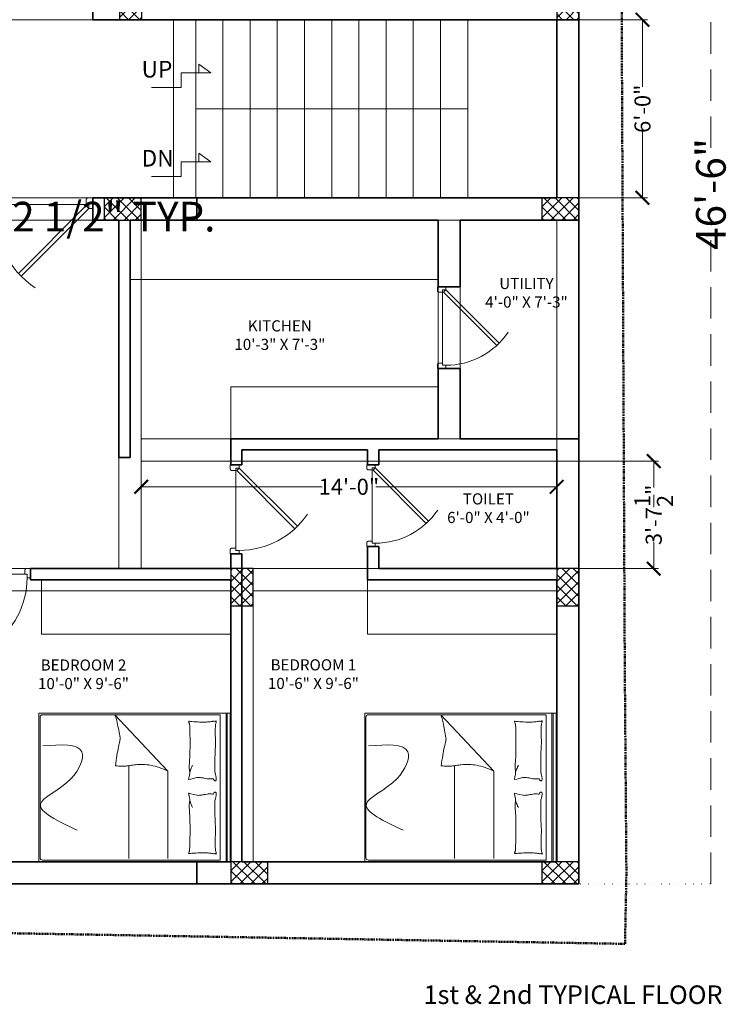
# Model space of a CAD drawing. Units: inches. Extents: x -16911 to -9621, y -48626 to -46270.
# Tile 12 of 20: x -11965 to -11678, y -46993 to -46595. Entities that reach past the tile are written whole.
import ezdxf

# ---------------------------------------------------------------- set-up
doc = ezdxf.new("R2010")
doc.units = ezdxf.units.IN
for name, pattern in [('DASHDOT', [1, 0.5, -0.25, 0, -0.25]), ('DASHED', [19.05, 12.7, -6.35]), ('DOT2', [3.175, 0, -3.175])]:
    doc.linetypes.add(name, pattern=pattern)
for name, color, linetype, lineweight in [('A-ANNO-DIMS', 2, 'Continuous', 13), ('A-ANNO-SYMB', 3, 'Continuous', 13), ('A-ANNO-TEXT', 7, 'Continuous', 18), ('A-AREA-IDEN', 3, 'Continuous', 18), ('A-DOOR', 4, 'Continuous', 18), ('A-FLOR-STRS', 3, 'Continuous', 18), ('A-FURN', 8, 'Continuous', 13), ('A-WALL', 7, 'Continuous', 35), ('C-PROP', 6, 'DASHDOT', 50), ('column', 12, 'Continuous', 30), ('DOOR', 143, 'Continuous', 9), ('EXT BEAM', 132, 'Continuous', 13), ('furniture', 35, 'Continuous', 15), ('S-BEAM', 132, 'Continuous', 25), ('S-COLS', 1, 'Continuous', 30), ('STAIRCASE', 137, 'Continuous', 5)]:
    doc.layers.add(name, color=color, linetype=linetype, lineweight=lineweight)
doc.styles.get("Standard").update_dxf_attribs({"font": 'swissel.ttf'})
doc.styles.add('style3', font='times.ttf')
doc.styles.add('style9', font='swisscl.ttf', dxfattribs={"height": 12})
doc.dimstyles.new('Dim9', dxfattribs={"dimtxt": 10, "dimasz": 0.199219, "dimexe": 1, "dimexo": 0.5, "dimgap": 1, "dimtad": 0, "dimdec": 1, "dimzin": 0, "dimdsep": 46, "dimlunit": 4, "dimtxsty": 'style9', "dimblk": 'ARCHTICK', "dimcen": 0.09, "dimclrd": 256, "dimclrt": 256, "dimadec": 0, "dimazin": 0, "dimtfac": 1, "dimtdec": 1, "dimtix": 1, "dimtofl": 0, "dimtmove": 1, "dimatfit": 3, "dimfxl": 9, "dimtolj": 1, "dimtzin": 0, "dimlwd": -1, "dimarcsym": 0})
doc.dimstyles.new('S.S.S', dxfattribs={"dimtxt": 6.5, "dimasz": 5.5, "dimexe": 2, "dimexo": 0, "dimgap": 0.09, "dimtad": 0, "dimdec": 1, "dimzin": 3, "dimdsep": 46, "dimlunit": 4, "dimtxsty": 'style3', "dimblk": 'ARCHTICK', "dimcen": 2.5, "dimclrd": 252, "dimclre": 256, "dimclrt": 7, "dimadec": 0, "dimazin": 0, "dimtfac": 1, "dimtdec": 1, "dimtix": 1, "dimtofl": 0, "dimtmove": 0, "dimatfit": 3, "dimfxl": 2, "dimtolj": 1, "dimtzin": 0, "dimlwd": 13, "dimlwe": 15, "dimarcsym": 0})

# ---------------------------------------------------------------- blocks, each defined once
blk = doc.blocks.new('hjuyuiuyk')
at = {"layer": 'furniture'}
for p, q in [((-19327.49, -39738.98), (-19327.49, -39737.31)), ((-19327.49, -39737.31), (-19267.49, -39737.31, 0)), ((-19327.49, -39746.54), (-19327.49, -39737.31)), ((-19267.49, -39738.5), (-19327.49, -39738.5, 0)), ((-19327.49, -39738.5, 0), (-19327.49, -39814.72, 0)), ((-19327.49, -39738.5), (-19327.49, -39814.72)), ((-19267.49, -39738.5, 0), (-19327.49, -39738.5)), ((-19267.49, -39738.98, 0), (-19327.49, -39738.98)), ((-19267.49, -39737.31, 0), (-19267.49, -39738.98, 0)), ((-19267.49, -39746.54, 0), (-19267.49, -39737.31, 0)), ((-19267.49, -39814.72), (-19267.49, -39738.5)), ((-19267.49, -39814.72, 0), (-19267.49, -39738.5, 0)), ((-19268.1, -39741.33), (-19326.9, -39741.33)), ((-19326.9, -39741.33), (-19326.9, -39813.21)), ((-19268.1, -39813.21), (-19268.1, -39741.33)), ((-19300.88, -39753.22, 0), (-19301.49, -39750.81, 0)), ((-19294.97, -39753.22, 0), (-19294.37, -39750.81, 0)), ((-19300.67, -39754.09, 0), (-19300.88, -39753.22, 0)), ((-19295.19, -39754.09, 0), (-19294.97, -39753.22, 0)), ((-19304.07, -39762.52), (-19326.9, -39783.91)), ((-19304.07, -39762.52), (-19268.82, -39762.52)), ((-19268.82, -39778.34), (-19306.29, -39778.34)), ((-19326.9, -39813.21), (-19326.9, -39783.91)), ((-19327.49, -39814.72, 0), (-19267.49, -39814.72)), ((-19327.49, -39814.72), (-19267.49, -39814.72, 0)), ((-19269.1, -39814.21), (-19325.9, -39814.21)), ((-19325.9, -39814.21), (-19269.1, -39814.21))]:
    blk.add_line(p, q, dxfattribs=at)
for centre, radius, start, end in [((-19324.36, -39743.07, 0), 0.0997, 111.7883, 160.436), ((-19324.39, -39743.06, 0), 0.0676, 160.436, 281.8931), ((-19324.12, -39743.66, 0), 0.732, 94.3025, 111.7883), ((-19324.35, -39743.25, 0), 0.125, 21.9904, 101.8931), ((-19323.34, -39743.89, 0), 0.956, 158.579, 188.1335), ((-19317.18, -39743.01, 0), 7.17, 188.1335, 192.1095), ((-19324.65, -39743.37, 0), 0.455, 338.579, 21.9904), ((-19329.85, -39745.73, 0), 5.78, 7.6809, 12.1095), ((-19324.11, -39743.77, 0), 0.842, 59.3487, 94.3025), ((-19322.88, -39741.69, 0), 1.57, 239.3487, 264.7408), ((-19319.6, -39692.5, 0), 50.87, 266.1399, 268.6002), ((-19319.84, -39713.09, 0), 30.28, 268.0921, 271.2808), ((-19320.24, -39695.07, 0), 48.31, 271.2808, 273.4034), ((-19316.15, -39763.89, 0), 20.63, 90.1553, 93.4034), ((-19316.09, -39783.15, 0), 39.89, 86.9902, 90.1553), ((-19305.86, -39588.51, 0), 155.02, 266.9902, 268.5957), ((-19305.42, -39570.46, 0), 173.07, 268.5957, 270), ((-19305.42, -39718.38, 0), 25.15, 270, 273.6841), ((-19304.03, -39739.9, 0), 3.58, 273.6841, 287.1951), ((-19300.46, -39751.46, 0), 8.51, 98.4372, 107.1951), ((-19301.02, -39747.69, 0), 4.7, 90, 98.4372), ((-19301.12, -39743.14, 0), 0.997, 274.4002, 333.4195), ((-19315.3, -39745.68, 0), 14.34, 360, 6.2324), ((-19301.02, -39745.63, 0), 2.64, 78.7276, 90), ((-19300.58, -39743.42, 0), 0.383, 333.4195, 78.7276), ((-19295.28, -39743.42, 0), 0.383, 101.2724, 206.5805), ((-19294.73, -39743.14, 0), 0.997, 206.5805, 265.5998), ((-19294.84, -39745.63, 0), 2.64, 90, 101.2724), ((-19280.55, -39745.68, 0), 14.34, 173.7676, 180), ((-19294.84, -39747.69, 0), 4.7, 81.5628, 90), ((-19295.39, -39751.46, 0), 8.51, 72.8049, 81.5628), ((-19291.82, -39739.9, 0), 3.58, 252.8049, 266.3159), ((-19290.43, -39718.38, 0), 25.15, 266.3159, 270), ((-19290.43, -39570.46, 0), 173.07, 270, 271.4043), ((-19289.99, -39588.51, 0), 155.02, 271.4043, 273.0098), ((-19279.76, -39783.15, 0), 39.89, 89.8447, 93.0098), ((-19279.7, -39763.89, 0), 20.63, 86.5966, 89.8447), ((-19275.61, -39695.07, 0), 48.31, 266.5966, 268.7192), ((-19276.02, -39713.09, 0), 30.28, 268.7192, 271.9079), ((-19276.73, -39645.13, 0), 98.25, 271.0069, 272.7772), ((-19272.12, -39741.69, 0), 1.57, 275.2592, 300.6513), ((-19270.89, -39743.77, 0), 0.842, 85.6975, 120.6513), ((-19265.15, -39745.73, 0), 5.78, 167.8905, 172.3191), ((-19270.88, -39743.66, 0), 0.732, 68.2117, 85.6975), ((-19270.35, -39743.37, 0), 0.455, 158.0096, 201.421), ((-19277.82, -39743.01, 0), 7.17, 347.8905, 351.8665), ((-19270.65, -39743.25, 0), 0.125, 78.1069, 158.0096), ((-19271.66, -39743.89, 0), 0.956, 351.8665, 21.421), ((-19270.61, -39743.06, 0), 0.0676, 258.1069, 19.564), ((-19270.64, -39743.07, 0), 0.0997, 19.564, 68.2117), ((-19350.51, -39748.51, 0), 26.62, 3.3687, 7.6809), ((-19343.69, -39748.11, 0), 19.79, 358.3669, 3.3687), ((-19282.35, -39751.13, 0), 19.21, 171.9949, 177.3351), ((-19292.22, -39749.75, 0), 9.25, 167.8016, 171.9949), ((-19326.4, -39742.36, 0), 25.72, 347.8016, 350.3156), ((-19306.91, -39745.68, 0), 5.95, 350.3156, 360), ((-19288.94, -39745.68, 0), 5.95, 180, 189.6844), ((-19269.45, -39742.36, 0), 25.72, 189.6844, 192.1984), ((-19303.63, -39749.75, 0), 9.25, 8.0051, 12.1984), ((-19313.5, -39751.13, 0), 19.21, 2.6649, 8.0051), ((-19251.31, -39748.11, 0), 19.79, 176.6313, 181.6331), ((-19244.49, -39748.51, 0), 26.62, 172.3191, 176.6313), ((-19720.99, -39728.47, 0), 397.61, 356.4951, 356.945), ((-19363.7, -39747.54, 0), 39.81, 356.945, 358.3669), ((-19299.57, -39750.33, 0), 1.97, 177.3351, 194.0452), ((-19296.28, -39750.33, 0), 1.97, 345.9548, 2.6649), ((-19231.3, -39747.54, 0), 39.81, 181.6331, 183.055), ((-18874.01, -39728.47, 0), 397.61, 183.055, 183.5049), ((-19323.69, -39753.93, 0), 0.564, 170.0016, 196.6978), ((-19333.47, -39752.21, 0), 9.37, 350.0016, 356.4951), ((-19324.19, -39754.08, 0), 0.0385, 196.6978, 277.1204), ((-19324.51, -39751.59, 0), 2.55, 277.1204, 286.2212), ((-19324.42, -39751.9, 0), 2.23, 286.2212, 297.4439), ((-19322.81, -39754.99, 0), 1.25, 102.448, 117.4439), ((-19322.32, -39757.22, 0), 3.54, 93.574, 102.448), ((-19318.44, -39837.61, 0), 84.03, 90.9755, 92.7955), ((-19315.55, -39952.16, 0), 198.61, 89.4461, 91.2473), ((-19314.9, -39885.06, 0), 131.51, 87.2326, 89.4461), ((-19310.57, -39795.48, 0), 41.81, 85.4012, 87.2326), ((-19304.32, -39717.78, 0), 36.14, 265.4012, 267.3712), ((-19297.32, -39733.09, 0), 21.54, 244.6889, 246.5156), ((-19305.66, -39747.05, 0), 6.83, 267.3712, 281.4827), ((-19297.32, -39733.09, 0), 21.54, 246.5156, 248.3423), ((-19297.32, -39733.09, 0), 21.54, 248.3423, 250.572), ((-19297.32, -39733.09, 0), 21.54, 250.572, 252.8018), ((-19303.46, -39757.91, 0), 4.25, 83.5659, 101.4827), ((-19303.37, -39757.16, 0), 3.49, 72.6136, 83.5659), ((-19300.33, -39747.43, 0), 6.7, 252.6136, 260.5159), ((-19300.13, -39746.25, 0), 7.9, 260.5159, 265.9171), ((-19300.69, -39754.1, 0), 0.0267, 265.9171, 14.0449), ((-19295.16, -39754.1, 0), 0.0267, 165.9551, 274.0829), ((-19295.72, -39746.25, 0), 7.9, 274.0829, 279.4841), ((-19295.52, -39747.43, 0), 6.7, 279.4841, 287.3864), ((-19292.48, -39757.16, 0), 3.49, 96.4341, 107.3864), ((-19292.39, -39757.91, 0), 4.25, 78.5173, 96.4341), ((-19298.54, -39733.09, 0), 21.54, 287.1982, 289.428), ((-19290.19, -39747.05, 0), 6.83, 258.5173, 272.6288), ((-19298.54, -39733.09, 0), 21.54, 289.428, 291.6577), ((-19298.54, -39733.09, 0), 21.54, 291.6577, 293.4844), ((-19298.54, -39733.09, 0), 21.54, 293.4844, 295.3111), ((-19291.53, -39717.78, 0), 36.14, 272.6288, 274.5988), ((-19285.28, -39795.48, 0), 41.81, 92.7674, 94.5988), ((-19280.95, -39885.06, 0), 131.51, 90.5539, 92.7674), ((-19280.3, -39952.16, 0), 198.61, 88.7527, 90.5539), ((-19277.1, -39805.01, 0), 51.42, 86.426, 88.7527), ((-19274.68, -39799.75, 0), 46.07, 86.5575, 89.0171), ((-19272.19, -39754.99, 0), 1.25, 62.5561, 77.552), ((-19270.58, -39751.9, 0), 2.23, 242.5561, 253.7788), ((-19270.49, -39751.59, 0), 2.55, 253.7788, 262.8796), ((-19261.53, -39752.21, 0), 9.37, 183.5049, 189.9984), ((-19270.81, -39754.08, 0), 0.0385, 262.8796, 343.3022), ((-19271.31, -39753.93, 0), 0.564, 343.3022, 9.9984), ((-19279.47, -39774.89), 27.53, 153.3084, 168.7423), ((-19287.94, -39773.2), 18.89, 168.7423, 187.3994), ((-19242.78, -39767.34), 64.43, 187.3994, 189.2719), ((-19333.07, -39782.08), 27.05, 6.3817, 9.2719), ((-19321.79, -39780.82), 15.7, 359.2313, 6.3817), ((-19306.77, -39846.83), 66.07, 105.9352, 107.7364), ((-19318.41, -39806.06), 23.67, 102.9255, 105.9352), ((-19287.64, -39956.87), 177.57, 99.7243, 101.7196), ((-19317.24, -39783.9), 2.09, 82.2696, 100.7276), ((-19317.9, -39788.76), 6.99, 76.8096, 82.2696), ((-19295.64, -39693.77), 90.57, 256.8096, 258.3259), ((-19295.11, -39691.23), 93.17, 258.3259, 260.505), ((-19288.03, -39648.9), 136.08, 260.505, 262.308), ((-19336.71, -39780.62), 30.63, 354.1141, 359.2313), ((-19325.9, -39813.21), 1, 180, 270), ((-19269.1, -39813.21), 1, 270, 0)]:
    blk.add_arc(centre, radius, start, end, dxfattribs=at)
blk.add_open_spline([(-19280.24, -39799.21), (-19283.87, -39806.94), (-19290.73, -39821.55), (-19298.08, -39801.09), (-19315.85, -39793.47), (-19314.86, -39805.92), (-19314.29, -39813.13)], degree=3, knots=[0, 0, 0, 0, 18.167809, 34.338432, 45.972904, 61.997799, 61.997799, 61.997799, 61.997799], dxfattribs=at)
blk = doc.blocks.new('A$C1C9D3E54')
at = {"layer": 'DOOR'}
blk.add_line((18676.53, 5780.72), (18710.53, 5780.72), dxfattribs=at)
blk.add_lwpolyline([(18685.01, 5806.62), (18710.47, 5781.16), (18711.53, 5782.22), (18686.07, 5807.68), (18685.01, 5806.62)], dxfattribs=at)
blk.add_lwpolyline([(18674.03, 5778.22), (18676.03, 5778.22), (18674.03, 5778.22), (18674.03, 5782.22), (18675.53, 5782.22), (18675.53, 5780.72), (18676.53, 5780.72), (18676.53, 5778.72), (18676.41, 5778.72), (18676.41, 5778.6, -0.414214), (18676.16, 5778.35), (18676.03, 5778.35), (18676.03, 5778.22)], format="xyb", dxfattribs=at)
blk.add_lwpolyline([(18713.03, 5782.22), (18711.53, 5782.22), (18711.53, 5780.72), (18710.53, 5780.72), (18710.53, 5778.72), (18710.66, 5778.72), (18710.66, 5778.6, 0.414214), (18710.91, 5778.35), (18711.03, 5778.35), (18711.03, 5778.22), (18713.03, 5778.22), (18711.03, 5778.22), (18713.03, 5778.22), (18713.03, 5782.22)], format="xyb", close=True, dxfattribs=at)
blk.add_arc((18711.53, 5782.22), 36, 124.0336, 180, dxfattribs=at)
blk = doc.blocks.new('THYHYTJ')
at = {"layer": 'STAIRCASE', "ltscale": 10}
for p, q in [((-7981.18, -46346.18), (-7984.62, -46351.1)), ((-7981.18, -46358.18), (-7981.18, -46346.18)), ((-7984.62, -46351.1), (-7981.18, -46351.1)), ((-7975.18, -46358.18), (-7981.18, -46358.18)), ((-7975.18, -46370.18), (-7975.18, -46358.18))]:
    blk.add_line(p, q, dxfattribs=at)
blk = doc.blocks.new('COLUMNS')
at = {"layer": 'column'}
h = blk.add_hatch(dxfattribs=at)
h.set_pattern_fill('ANSI37', color=256, angle=-720)
h.set_pattern_definition([(45, (21840.2088, -104675.1704), (-2.24506403, 2.24506403), []), (135, (21840.2088, -104675.1704), (-2.24506403, -2.24506403), [])])
h.paths.add_polyline_path([(-11924.72, -46595.36), (-11915.72, -46595.36), (-11915.72, -46580.36), (-11924.72, -46580.36)])
h = blk.add_hatch(dxfattribs=at)
h.set_pattern_fill('ANSI37', color=256, angle=-900)
h.set_pattern_definition([(225, (-45503.8578, 11499.4594), (2.24506403, -2.24506403), []), (315, (-45503.8578, 11499.4594), (2.24506403, 2.24506403), [])])
h.paths.add_polyline_path([(-11738.92, -46580.36), (-11747.92, -46580.36), (-11747.92, -46595.36), (-11738.92, -46595.36)])
h = blk.add_hatch(dxfattribs=at)
h.set_pattern_fill('ANSI37', color=256, angle=-810)
h.set_pattern_definition([(315, (-70010.7892, -80432.2886), (2.24506403, 2.24506403), []), (45, (-70010.7892, -80432.2886), (-2.24506403, 2.24506403), [])])
h.paths.add_polyline_path([(-11930.97, -46667.36), (-11930.97, -46676.36), (-11915.97, -46676.36), (-11915.97, -46667.36)])
h = blk.add_hatch(dxfattribs=at)
h.set_pattern_fill('ANSI37', color=256, angle=-810)
h.set_pattern_definition([(315, (-69833.7395, -80432.2886), (2.24506403, 2.24506403), []), (45, (-69833.7395, -80432.2886), (-2.24506403, 2.24506403), [])])
h.paths.add_polyline_path([(-11753.92, -46667.36), (-11753.92, -46676.36), (-11738.92, -46676.36), (-11738.92, -46667.36)])
h = blk.add_hatch(dxfattribs=at)
h.set_pattern_fill('ANSI37', color=256, angle=-720)
h.set_pattern_definition([(45, (21885.2088, -104912.1242), (-2.24506403, 2.24506403), []), (135, (21885.2088, -104912.1242), (-2.24506403, -2.24506403), [])])
h.paths.add_polyline_path([(-11879.72, -46832.31), (-11870.72, -46832.31), (-11870.72, -46817.31), (-11879.72, -46817.31)])
h = blk.add_hatch(dxfattribs=at)
h.set_pattern_fill('ANSI37', color=256, angle=-720)
h.set_pattern_definition([(45, (22017.1023, -104912.1242), (-2.24506403, 2.24506403), []), (135, (22017.1023, -104912.1242), (-2.24506403, -2.24506403), [])])
h.paths.add_polyline_path([(-11747.83, -46832.31), (-11738.83, -46832.31), (-11738.83, -46817.31), (-11747.83, -46817.31)])
h = blk.add_hatch(dxfattribs=at)
h.set_pattern_fill('ANSI37', color=256, angle=-810)
h.set_pattern_definition([(315, (-69959.5392, -80700.7425), (2.24506403, 2.24506403), []), (45, (-69959.5392, -80700.7425), (-2.24506403, 2.24506403), [])])
h.paths.add_polyline_path([(-11879.72, -46935.81), (-11879.72, -46944.81), (-11864.72, -46944.81), (-11864.72, -46935.81)])
h = blk.add_hatch(dxfattribs=at)
h.set_pattern_fill('ANSI37', color=256, angle=-810)
h.set_pattern_definition([(315, (-69833.7395, -80700.7425), (2.24506403, 2.24506403), []), (45, (-69833.7395, -80700.7425), (-2.24506403, 2.24506403), [])])
h.paths.add_polyline_path([(-11753.92, -46935.81), (-11753.92, -46944.81), (-11738.92, -46944.81), (-11738.92, -46935.81)])
at = {"layer": 'column', "ltscale": 0.05}
for points in [[(-11915.72, -46580.36), (-11924.72, -46580.36), (-11924.72, -46595.36), (-11915.72, -46595.36)], [(-11747.92, -46595.36), (-11738.92, -46595.36), (-11738.92, -46580.36), (-11747.92, -46580.36)], [(-11915.97, -46676.36), (-11915.97, -46667.36), (-11930.97, -46667.36), (-11930.97, -46676.36)], [(-11738.92, -46676.36), (-11738.92, -46667.36), (-11753.92, -46667.36), (-11753.92, -46676.36)], [(-11870.72, -46817.31), (-11879.72, -46817.31), (-11879.72, -46832.31), (-11870.72, -46832.31)], [(-11738.83, -46817.31), (-11747.83, -46817.31), (-11747.83, -46832.31), (-11738.83, -46832.31)], [(-11864.72, -46944.81), (-11864.72, -46935.81), (-11879.72, -46935.81), (-11879.72, -46944.81)], [(-11738.92, -46944.81), (-11738.92, -46935.81), (-11753.92, -46935.81), (-11753.92, -46944.81)]]:
    blk.add_lwpolyline(points, close=True, dxfattribs=at)
blk = doc.blocks.new('TYPICAL BEAMS G-2')
at = {"layer": 'EXT BEAM'}
for p, q in [((-11738.92, -48216.7), (-11738.92, -47658.74)), ((-12052.47, -47867.24), (-11924.72, -47867.24)), ((-11915.72, -47867.24), (-11747.92, -47867.24)), ((-11902.92, -47867.24), (-11902.92, -47939.24)), ((-11893.92, -47867.24), (-11893.92, -47939.24)), ((-11747.92, -47939.24), (-11747.92, -47867.24)), ((-12046.47, -47939.24), (-11929.47, -47939.24)), ((-11920.47, -47939.24), (-11738.92, -47939.24)), ((-12046.47, -47948.24), (-11929.47, -47948.24)), ((-11924.97, -47948.24), (-11924.97, -48089.2)), ((-11920.47, -47948.24), (-11738.92, -47948.24)), ((-11915.97, -47948.24), (-11915.97, -48089.2)), ((-11795.92, -47948.24), (-11795.92, -48036.7)), ((-11786.92, -47948.24), (-11786.92, -48036.7)), ((-11747.92, -48089.2), (-11747.92, -47948.24)), ((-11747.92, -48036.7), (-11915.97, -48036.7)), ((-11747.92, -48045.7), (-11915.97, -48045.7)), ((-12052.47, -48089.2), (-11747.92, -48089.2)), ((-12052.47, -48098.2), (-11879.72, -48098.2)), ((-11879.72, -48098.2), (-11879.72, -48207.7)), ((-11870.72, -48098.2), (-11747.92, -48098.2)), ((-11870.72, -48098.2), (-11870.72, -48207.7)), ((-11747.92, -48207.7), (-11747.92, -48098.2)), ((-12052.47, -48207.7), (-11879.72, -48207.7)), ((-11870.72, -48207.7), (-11747.92, -48207.7)), ((-12061.47, -48216.7), (-11738.92, -48216.7))]:
    blk.add_line(p, q, dxfattribs=at)
blk = doc.blocks.new('_ArchTick')
at = {"color": 0, "linetype": 'ByBlock', "const_width": 0.15}
blk.add_lwpolyline([(-0.5, -0.5), (0.5, 0.5)], dxfattribs=at)
blk = doc.blocks.new('*D32')
at = {"layer": 'A-ANNO-DIMS', "color": 0, "lineweight": 15, "transparency": 16777216}
for p, q in [((-11747.92, -46595.36), (-11711.23, -46595.36)), ((-11746.42, -46667.36), (-11711.23, -46667.36))]:
    blk.add_line(p, q, dxfattribs=at)
at = {"layer": 'A-ANNO-DIMS', "color": 0, "lineweight": 13, "transparency": 16777216}
for p, q in [((-11713.23, -46595.36), (-11713.23, -46622.57)), ((-11713.23, -46667.36), (-11713.23, -46640.14))]:
    blk.add_line(p, q, dxfattribs=at)
at = {"layer": 'Defpoints', "color": 0, "transparency": 16777216}
for p in [(-11747.92, -46595.36), (-11713.23, -46595.36), (-11746.42, -46667.36)]:
    blk.add_point(p, dxfattribs=at)
at = {"layer": 'A-ANNO-DIMS', "color": 0, "lineweight": 13, "transparency": 16777216, "xscale": 5.5, "yscale": 5.5, "zscale": 5.5}
for p, rotation in [((-11713.23, -46595.36), 90), ((-11713.23, -46667.36), 270)]:
    blk.add_blockref('_ArchTick', p, dxfattribs=dict(at, rotation=rotation))
at = {"layer": 'A-ANNO-DIMS', "color": 0, "transparency": 16777216, "insert": (-11713.23, -46631.36), "char_height": 6.5, "attachment_point": 5, "rotation": 90, "style": 'style3'}
blk.add_mtext('\\A1;6\'-0"', dxfattribs=at)
blk = doc.blocks.new('*D40')
at = {"layer": 'A-ANNO-DIMS', "color": 0, "lineweight": 15, "transparency": 16777216}
for p, q in [((-11747.92, -46773.81), (-11706.69, -46773.81)), ((-11747.92, -46817.31), (-11706.69, -46817.31))]:
    blk.add_line(p, q, dxfattribs=at)
at = {"layer": 'A-ANNO-DIMS', "color": 0, "lineweight": 13, "transparency": 16777216}
for p, q in [((-11708.69, -46773.81), (-11708.69, -46784.49)), ((-11708.69, -46817.31), (-11708.69, -46806.62))]:
    blk.add_line(p, q, dxfattribs=at)
at = {"layer": 'Defpoints', "color": 0, "transparency": 16777216}
for p in [(-11747.92, -46773.81), (-11747.92, -46817.31), (-11708.69, -46817.31)]:
    blk.add_point(p, dxfattribs=at)
at = {"layer": 'A-ANNO-DIMS', "color": 0, "lineweight": 13, "transparency": 16777216, "xscale": 5.5, "yscale": 5.5, "zscale": 5.5}
for p, rotation in [((-11708.69, -46773.81), 90), ((-11708.69, -46817.31), 270)]:
    blk.add_blockref('_ArchTick', p, dxfattribs=dict(at, rotation=rotation))
at = {"layer": 'A-ANNO-DIMS', "color": 0, "transparency": 16777216, "insert": (-11708.69, -46795.56), "char_height": 6.5, "attachment_point": 5, "rotation": 90, "style": 'style3'}
blk.add_mtext('\\A1;3\'-7{\\H1x;\\S1/2;}"', dxfattribs=at)
blk = doc.blocks.new('*D41')
at = {"layer": 'A-ANNO-DIMS', "color": 0, "lineweight": 15, "transparency": 16777216}
for p, q in [((-11915.97, -46773.81), (-11915.97, -46786.22)), ((-11747.92, -46773.81), (-11747.92, -46786.22))]:
    blk.add_line(p, q, dxfattribs=at)
at = {"layer": 'A-ANNO-DIMS', "color": 0, "lineweight": 13, "transparency": 16777216}
for p, q in [((-11915.97, -46784.22), (-11842.78, -46784.22)), ((-11747.92, -46784.22), (-11821.12, -46784.22))]:
    blk.add_line(p, q, dxfattribs=at)
at = {"layer": 'Defpoints', "color": 0, "transparency": 16777216}
for p in [(-11915.97, -46773.81), (-11747.92, -46773.81), (-11915.97, -46784.22)]:
    blk.add_point(p, dxfattribs=at)
at = {"layer": 'A-ANNO-DIMS', "color": 0, "lineweight": 13, "transparency": 16777216, "xscale": 5.5, "yscale": 5.5, "zscale": 5.5, "rotation": 180}
blk.add_blockref('_ArchTick', (-11915.97, -46784.22), dxfattribs=at)
at = {"layer": 'A-ANNO-DIMS', "color": 0, "lineweight": 13, "transparency": 16777216, "xscale": 5.5, "yscale": 5.5, "zscale": 5.5}
blk.add_blockref('_ArchTick', (-11747.92, -46784.22), dxfattribs=at)
at = {"layer": 'A-ANNO-DIMS', "color": 0, "transparency": 16777216, "insert": (-11831.95, -46784.22), "char_height": 6.5, "attachment_point": 5, "style": 'style3'}
blk.add_mtext('\\A1;14\'-0"', dxfattribs=at)
blk = doc.blocks.new('*D75')
at = {"layer": 'A-ANNO-DIMS', "linetype": 'DASHED', "transparency": 16777216}
for p, q in [((-12016.12, -46674.98), (-12016.32, -46674.98)), ((-11977.71, -46674.98), (-11977.51, -46674.98))]:
    blk.add_line(p, q, dxfattribs=at)
at = {"layer": 'A-ANNO-DIMS', "color": 0, "linetype": 'DOT2', "lineweight": -2, "transparency": 16777216}
for p, q in [((-12016.12, -46680.24), (-12016.12, -46673.98)), ((-11977.71, -46680.24), (-11977.71, -46673.98))]:
    blk.add_line(p, q, dxfattribs=at)
at = {"layer": 'Defpoints', "color": 0, "transparency": 16777216}
for p in [(-11977.71, -46674.98), (-12016.12, -46680.74), (-11977.71, -46680.74)]:
    blk.add_point(p, dxfattribs=at)
at = {"layer": 'A-ANNO-DIMS', "transparency": 16777216, "xscale": 0.19921875, "yscale": 0.19921875, "zscale": 0.19921875}
blk.add_blockref('_ArchTick', (-12016.12, -46674.98), dxfattribs=at)
at = {"layer": 'A-ANNO-DIMS', "transparency": 16777216, "xscale": 0.19921875, "yscale": 0.19921875, "zscale": 0.19921875, "rotation": 180}
blk.add_blockref('_ArchTick', (-11977.71, -46674.98), dxfattribs=at)
at = {"layer": 'A-ANNO-DIMS', "transparency": 16777216, "insert": (-11996.91, -46674.98), "char_height": 12, "attachment_point": 5, "style": 'style9'}
blk.add_mtext('\\A1;LOUNGE CHAIR 3\'-2 1/2" TYP.', dxfattribs=at)
blk = doc.blocks.new('*D115')
at = {"layer": 'A-ANNO-DIMS', "color": 0, "linetype": 'DOT2', "lineweight": -2, "transparency": 16777216}
for p, q in [((-11738.42, -46386.86), (-11684.58, -46386.86)), ((-11738.42, -46944.81), (-11684.58, -46944.81))]:
    blk.add_line(p, q, dxfattribs=at)
at = {"layer": 'A-ANNO-DIMS', "linetype": 'DASHED', "transparency": 16777216}
for p, q in [((-11685.58, -46386.86), (-11685.58, -46648.2)), ((-11685.58, -46944.81), (-11685.58, -46683.47))]:
    blk.add_line(p, q, dxfattribs=at)
at = {"layer": 'Defpoints', "color": 0, "transparency": 16777216}
for p in [(-11738.92, -46386.86), (-11738.92, -46944.81), (-11685.58, -46944.81)]:
    blk.add_point(p, dxfattribs=at)
at = {"layer": 'A-ANNO-DIMS', "transparency": 16777216, "xscale": 0.19921875, "yscale": 0.19921875, "zscale": 0.19921875}
for p, rotation in [((-11685.58, -46386.86), 90), ((-11685.58, -46944.81), 270)]:
    blk.add_blockref('_ArchTick', p, dxfattribs=dict(at, rotation=rotation))
at = {"layer": 'A-ANNO-DIMS', "transparency": 16777216, "insert": (-11685.58, -46665.83), "char_height": 12, "attachment_point": 5, "rotation": 90, "style": 'style9'}
blk.add_mtext('\\A1;46\'-6"', dxfattribs=at)

msp = doc.modelspace()

# ---------------------------------------------------------------- linework, layer by layer
at = {"layer": 'A-FLOR-STRS', "ltscale": 10}
for p, q in [((-11893.925, -46595.355), (-11893.925, -46667.355)), ((-11882.925, -46595.355), (-11882.925, -46667.355)), ((-11871.925, -46595.355), (-11871.925, -46667.355)), ((-11860.925, -46595.355), (-11860.925, -46667.355)), ((-11849.925, -46595.355), (-11849.925, -46667.355)), ((-11838.925, -46595.355), (-11838.925, -46667.355)), ((-11827.925, -46595.355), (-11827.925, -46667.355)), ((-11816.925, -46595.355), (-11816.925, -46667.355)), ((-11805.925, -46595.355), (-11805.925, -46667.355)), ((-11794.925, -46595.355), (-11794.925, -46667.355)), ((-11783.925, -46595.355), (-11783.925, -46667.355)), ((-11783.925, -46631.355), (-11893.925, -46631.355))]:
    msp.add_line(p, q, dxfattribs=at)
at = {"layer": 'A-FURN', "ltscale": 0.2}
for p, q in [((-11795.925, -46700.355), (-11920.474, -46700.355)), ((-11795.925, -46743.809), (-11879.724, -46743.809)), ((-11879.724, -46764.809), (-11879.724, -46743.809)), ((-11956.224, -46821.809, 0), (-11956.224, -46843.809, 0)), ((-11824.425, -46821.809), (-11824.425, -46843.809)), ((-11879.724, -46843.809), (-11956.224, -46843.809)), ((-11824.425, -46843.809), (-11747.925, -46843.809))]:
    msp.add_line(p, q, dxfattribs=at)
at = {"layer": 'A-WALL'}
for p, q in [((-11738.925, -46469.355), (-11738.925, -46676.355)), ((-11935.474, -46595.355), (-11935.474, -46586.355)), ((-11738.925, -46595.355), (-11935.474, -46595.355)), ((-11747.925, -46595.355), (-11747.925, -46667.355)), ((-11747.925, -46667.355), (-11935.474, -46667.355)), ((-11935.474, -46676.355), (-11935.474, -46667.355)), ((-11893.506, -46667.355), (-11893.506, -46676.355)), ((-11738.925, -46667.355), (-11738.925, -46676.355)), ((-11924.974, -46676.355), (-11935.474, -46676.355)), ((-11924.974, -46676.355), (-11924.974, -46772.355)), ((-11795.925, -46676.355), (-11920.474, -46676.355)), ((-11920.474, -46676.355), (-11920.474, -46772.355)), ((-11795.925, -46676.355), (-11795.925, -46703.355)), ((-11738.925, -46676.355), (-11786.925, -46676.355)), ((-11786.925, -46676.355), (-11786.925, -46703.355)), ((-11738.925, -46676.355), (-11738.925, -46764.809)), ((-11795.925, -46703.355), (-11786.925, -46703.355)), ((-11795.925, -46736.355), (-11795.925, -46764.809)), ((-11795.925, -46736.355), (-11786.925, -46736.355)), ((-11786.925, -46736.355), (-11786.925, -46764.809)), ((-11879.724, -46775.309), (-11879.724, -46764.809)), ((-11879.724, -46764.809), (-11795.925, -46764.809)), ((-11786.925, -46764.809), (-11738.925, -46764.809)), ((-11738.925, -46764.809), (-11738.925, -46944.809)), ((-11875.224, -46775.309), (-11875.224, -46769.309)), ((-11875.224, -46769.309), (-11824.425, -46769.309)), ((-11824.425, -46769.309), (-11824.425, -46775.309)), ((-11819.925, -46769.309), (-11819.925, -46775.309)), ((-11819.925, -46769.309), (-11747.925, -46769.309)), ((-11747.925, -46769.309), (-11747.925, -46817.309)), ((-11920.474, -46772.355), (-11924.974, -46772.355)), ((-11879.724, -46775.309), (-11875.224, -46775.309)), ((-11824.425, -46775.309), (-11819.925, -46775.309)), ((-11824.425, -46808.309), (-11824.425, -46821.809)), ((-11824.425, -46808.309), (-11819.925, -46808.309)), ((-11819.925, -46808.309), (-11819.925, -46817.309)), ((-11879.724, -46817.309), (-11879.724, -46811.309)), ((-11879.724, -46811.309), (-11875.224, -46811.309)), ((-11875.224, -46935.809), (-11875.224, -46811.309)), ((-11960.724, -46817.309), (-11879.724, -46817.309)), ((-11960.724, -46821.809), (-11960.724, -46817.309)), ((-11819.925, -46817.309), (-11747.925, -46817.309)), ((-11960.724, -46821.809), (-11879.724, -46821.809)), ((-11879.724, -46935.809), (-11879.724, -46821.809)), ((-11824.425, -46821.809), (-11747.925, -46821.809)), ((-11747.925, -46821.809), (-11747.925, -46935.809)), ((-11999.974, -46935.809), (-11879.724, -46935.809)), ((-11893.506, -46935.809), (-11893.506, -46944.809)), ((-11875.224, -46935.809), (-11747.925, -46935.809)), ((-11738.925, -46935.809), (-11738.925, -46944.809)), ((-12008.974, -46944.809), (-11738.925, -46944.809))]:
    msp.add_line(p, q, dxfattribs=at)
at = {"layer": 'C-PROP'}
msp.add_lwpolyline([(-12080.474, -46962.809), (-11720.293, -46969.035), (-11719.732, -46940.446), (-11720.395, -46855.606), (-11721.561, -46609.511), (-11721.175, -46367.855), (-12080.838, -46362.811), (-12080.3, -46762.955)], close=True, dxfattribs=at)

# ---------------------------------------------------------------- block references
at = {"layer": 'A-ANNO-SYMB', "rotation": 270.0000000000144}
for p in [(34458.429, -54597.957), (34458.429, -54633.957)]:
    msp.add_blockref('THYHYTJ', p, dxfattribs=at)
at = {"layer": 'A-DOOR'}
for p, xscale, yscale, zscale, rotation in [((-32087.969, -40444.653), -1.076923076922859, 1.076923076922859, 1.076923076922859, 180), ((-16685.441, -62537.458), -0.8461538461538624, 0.8461538461538624, 0.8461538461538624, 270), ((-17213.72, -64048.876), -0.9230769230769229, 0.9230769230769229, 0.9230769230769229, 270), ((-16713.941, -62609.412), -0.8461538461538624, 0.8461538461538624, 0.8461538461538624, 270), ((5276.842, -41483.564), 0.9230769230769229, 0.9230769230769229, 0.9230769230769229, 180)]:
    msp.add_blockref('A$C1C9D3E54', p, dxfattribs=dict(at, xscale=xscale, yscale=yscale, zscale=zscale, rotation=rotation))
at = {"layer": 'A-FURN', "rotation": 270}
for p in [(27857.338, -66203.296), (27989.137, -66203.296, 0)]:
    msp.add_blockref('hjuyuiuyk', p, dxfattribs=at)
at = {"layer": 'S-BEAM'}
msp.add_blockref('TYPICAL BEAMS G-2', (0, 1271.886), dxfattribs=at)
at = {"layer": 'S-COLS'}
msp.add_blockref('COLUMNS', (0, 0), dxfattribs=at)

# ---------------------------------------------------------------- texts
at = {"layer": 'A-ANNO-TEXT'}
for s, p in [('UP', (-11915.824, -46618.742)), ('DN', (-11915.824, -46654.742))]:
    msp.add_text(s, height=6.75, dxfattribs=at).set_placement(p)
at = {"layer": 'A-ANNO-TEXT', "ltscale": 10, "insert": (-11801.781, -46985.845), "char_height": 7.5, "width": 166.78033, "attachment_point": 1, "style": 'style9'}
msp.add_mtext('\\A1;{\\fCentury Gothic|b0|i0|c0|p34;1st & 2nd TYPICAL FLOOR}', dxfattribs=at)
at = {"layer": 'A-AREA-IDEN', "ltscale": 10, "char_height": 4.5, "width": 42.823, "attachment_point": 1, "style": 'style9'}
for s, insert in [('\\A1;\\pxqc;{\\fCentury Gothic|b0|i0|c0|p34;UTILITY\\P4\'-0" X 7\'-3"}', (-11781.564, -46699.772)), ('\\A1;\\pxqc;{\\fCentury Gothic|b0|i0|c0|p34;KITCHEN\\P10\'-3" X 7\'-3"}', (-11881.298, -46716.893)), ('\\A1;\\pxqc;{\\fCentury Gothic|b0|i0|c0|p34;TOILET\\P6\'-0" X 4\'-0"}', (-11796.951, -46786.873)), ('\\A1;\\pxqc;{\\fCentury Gothic|b0|i0|c0|p34;BEDROOM 2\\P10\'-0" X 9\'-6"}', (-11960.722, -46854.047)), ('\\A1;\\pxqc;{\\fCentury Gothic|b0|i0|c0|p34;BEDROOM 1\\P10\'-6" X 9\'-6"}', (-11867.728, -46853.971))]:
    msp.add_mtext(s, dxfattribs=dict(at, insert=insert))

# ---------------------------------------------------------------- dimensions: what is measured, and where the dimension line sits
at = {"layer": 'A-ANNO-DIMS'}
for base, p1, p2, dimstyle, override, picture, middle in [((-11685.582, -46944.809), (-11738.925, -46386.855), (-11738.925, -46944.809), 'Dim9', {"dimdec": 1, "dimlfac": 1, "dimrnd": 0, "dimzin": 1, "dimdsep": 46, "dimlunit": 4, "dimfrac": 2}, '*D115', (-11685.582, -46665.832)), ((-11713.234, -46595.355), (-11746.425, -46667.355), (-11747.925, -46595.355), 'S.S.S', {"dimclrd": 0, "dimclre": 0, "dimclrt": 0}, '*D32', (-11713.234, -46631.355)), ((-11708.694, -46817.309), (-11747.925, -46773.809), (-11747.925, -46817.309), 'S.S.S', {"dimclrd": 0, "dimclre": 0, "dimclrt": 0}, '*D40', (-11708.694, -46795.559))]:
    dim = msp.add_linear_dim(base=base, p1=p1, p2=p2, angle=90, dimstyle=dimstyle, override=override, dxfattribs=at)
    dim.commit()
    dim.dimension.update_dxf_attribs({"geometry": picture, "text_midpoint": middle})
dim = msp.add_linear_dim(base=(-11977.706, -46674.975), p1=(-12016.121, -46680.738), p2=(-11977.706, -46680.738), text='LOUNGE CHAIR <> TYP.', dimstyle='Dim9', override={"dimdec": 1, "dimrnd": 0, "dimzin": 1, "dimlunit": 4, "dimfrac": 2}, dxfattribs=at)
dim.commit()
dim.dimension.update_dxf_attribs({"geometry": '*D75', "text_midpoint": (-11996.914, -46674.975)})
dim = msp.add_linear_dim(base=(-11915.974, -46784.217), p1=(-11747.925, -46773.809), p2=(-11915.974, -46773.809), dimstyle='S.S.S', override={"dimclrd": 0, "dimclre": 0, "dimclrt": 0}, dxfattribs=at)
dim.commit()
dim.dimension.update_dxf_attribs({"geometry": '*D41', "text_midpoint": (-11831.949, -46784.217)})

doc.saveas('drawing.dxf')
